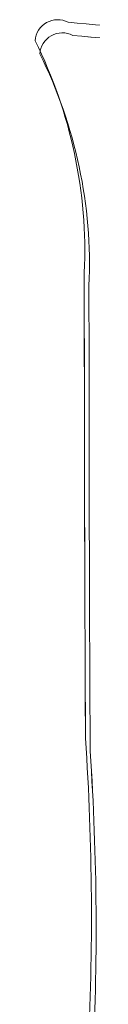
# Model space of a CAD drawing. Units: inches. Extents: x 1885 to 2748, y 783 to 2421.
# Tile 63 of 117: x 2046 to 2049, y 1920 to 1968. Entities that reach past the tile are written whole.
import ezdxf

# ---------------------------------------------------------------- set-up
doc = ezdxf.new("R2010")
doc.units = ezdxf.units.IN
doc.layers.add('A-FURN', color=8, linetype='Continuous', lineweight=13)

# ---------------------------------------------------------------- blocks, each defined once
blk = doc.blocks.new('BED-DOUBLE')
for centre, radius, start, end in [((69.309, 76.384), 23.065, 267.4714, 296.4681), ((69.309, 76.384), 23.065, 267.4714, 296.4681), ((79.513, 54.637), 1.102, 332.6588, 86.02), ((79.513, 54.637), 1.102, 332.6588, 86.02), ((68.67, 76.156), 23.065, 267.4714, 296.4681), ((68.67, 76.156), 23.065, 267.4714, 296.4681), ((78.874, 54.409), 1.102, 332.6588, 86.02), ((78.874, 54.408), 1.102, 332.6588, 86.02), ((212.28, 41.151), 133.04, 174.4998, 180.63509), ((212.28, 41.15), 133.04, 174.4998, 180.63509), ((212.92, 41.379), 133.04, 174.4998, 180.63509), ((212.92, 41.379), 133.04, 174.4998, 180.63509), ((36.958, 182.493), 129.499, 266.97912, 273.83645), ((36.958, 182.493), 129.499, 266.97912, 273.83645), ((68.464, -4508.516), 4561.858, 90.002168, 90.286887), ((68.464, -4508.517), 4561.858, 90.002168, 90.286887), ((36.319, 182.265), 129.499, 266.97912, 273.83645), ((36.319, 182.264), 129.499, 266.97912, 273.83645), ((67.825, -4508.745), 4561.858, 90.002168, 90.286887), ((67.825, -4508.745), 4561.858, 90.002168, 90.286887)]:
    blk.add_arc(centre, radius, start, end)

msp = doc.modelspace()

# ---------------------------------------------------------------- block references
at = {"layer": 'A-FURN', "rotation": 89.9999998331857}
msp.add_blockref('BED-DOUBLE', (2102.136, 1887.416), dxfattribs=at)

doc.saveas('drawing.dxf')
